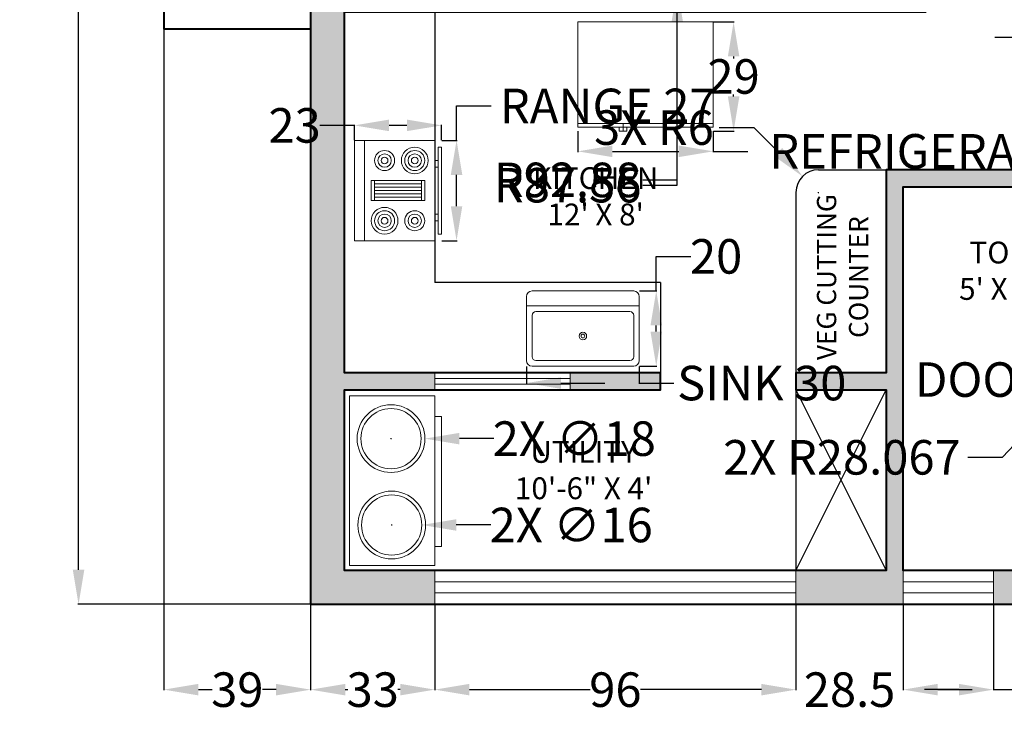
# Model space of a CAD drawing. Units: inches. Extents: x -51 to 563, y -59 to 453.
# Tile 1 of 6: x -51 to 211, y -59 to 125. Entities that reach past the tile are written whole.
import ezdxf

# ---------------------------------------------------------------- set-up
doc = ezdxf.new("R2010")
doc.units = ezdxf.units.IN
doc.header["$MEASUREMENT"] = 0
for name, color, linetype, lineweight in [('A-ANNO-DIMS', 2, 'Continuous', 18), ('A-ANNO-TEXT', 7, 'Continuous', 18), ('A-AREA-IDEN', 7, 'Continuous', 25), ('A-EQPM', 8, 'Continuous', 18), ('A-FLOR-CASE', 8, 'Continuous', 25), ('A-FLOR-FIXT', 9, 'Continuous', 18), ('A-GLAZ', 4, 'Continuous', 18), ('A-WALL', 7, 'Continuous', 40), ('A-WALL-PATT', 252, 'Continuous', 13)]:
    doc.layers.add(name, color=color, linetype=linetype, lineweight=lineweight)
doc.styles.get("Standard").update_dxf_attribs({"font": 'arial.ttf'})
doc.dimstyles.get("Standard").update_dxf_attribs({"dimtxt": 9.18, "dimasz": 9.18, "dimexe": 0.18, "dimexo": 0.0625, "dimgap": 0.09, "dimtad": 0, "dimtih": 1, "dimtoh": 1, "dimdec": 1, "dimzin": 0, "dimdsep": 46, "dimlunit": 3, "dimtxsty": 'Standard', "dimcen": 0.09, "dimadec": 0, "dimazin": 0, "dimtfac": 1, "dimtdec": 1, "dimtofl": 0, "dimtmove": 0, "dimatfit": 3, "dimfxl": 1, "dimtolj": 1, "dimtzin": 0, "dimarcsym": 0})

# ---------------------------------------------------------------- blocks, each defined once
blk = doc.blocks.new('Range-Oven - 30 in top')
for p, q in [((0, -3), (30, -3)), ((12, -6), (18, -6)), ((13, -20), (13, -6)), ((14, -6), (14, -20)), ((15, -20), (15, -6)), ((16, -6), (16, -20)), ((17, -20), (17, -6)), ((18, -20), (12, -20)), ((6, -24), (6, -25)), ((8, -25), (8, -24)), ((22, -25), (22, -24)), ((24, -24), (24, -25))]:
    blk.add_line(p, q)
for points in [[(0, -24), (0, 0), (30, 0), (30, -24)], [(12, -21), (12, -5), (18, -5), (18, -21)], [(2, -26), (2, -25), (28, -25), (28, -26)]]:
    blk.add_lwpolyline(points, close=True)
for centre, radius in [((6, -9), 4), ((6, -9), 3), ((6, -9), 2), ((6, -9), 1), ((24, -9), 3), ((24, -9), 2), ((24, -9), 1), ((24, -18), 4), ((6, -18), 3), ((6, -18), 2), ((6, -18), 1), ((24, -18), 3), ((24, -18), 2), ((24, -18), 1)]:
    blk.add_circle(centre, radius)
blk = doc.blocks.new('Sink-single - 30 in top')
blk.add_line((-15, -3.999996), (15, -3.999996))
for points in [[(-13.5, 0), (13.5, 0)], [(-15, -18.499996), (-15, -1.5)], [(15, -1.5), (15, -18.499996)], [(-13.5, -17.499996), (-13.5, -6.499996)], [(-12.5, -5.499996), (12.5, -5.499996)], [(13.5, -6.499996), (13.5, -17.499996)], [(13.5, -19.999996), (-13.5, -19.999996)], [(12.5, -18.499996), (-12.5, -18.499996)]]:
    blk.add_lwpolyline(points)
for radius in [1, 0.5]:
    blk.add_circle((0, -11.999996), radius)
for centre, radius, start, end in [((-13.5, -1.5), 1.5, 90, 180), ((13.5, -1.5), 1.5, 0, 90), ((-12.5, -6.499996), 1, 90, 180), ((12.5, -6.499996), 1, 0, 90), ((-12.5, -17.499996), 1, 180, 270), ((12.5, -17.499996), 1, 270, 0), ((-13.5, -18.499996), 1.5, 180, 270), ((13.5, -18.499996), 1.5, 270, 0)]:
    blk.add_arc(centre, radius, start, end)
blk = doc.blocks.new('Refrigerator-2 door - 36 in top')
for p, q in [((0, -26.999999), (36, -26.999999)), ((11, -27.999999), (11, -28.999999)), ((12, -26.999999), (12, -28.999999)), ((13, -28.999999), (13, -27.999999)), ((11, -28.999999), (13, -28.999999))]:
    blk.add_line(p, q)
blk.add_lwpolyline([(0, -27.999999), (0, 0), (36, 0), (36, -27.999999)], close=True)
blk = doc.blocks.new('*D43')
at = {"layer": 'A-ANNO-DIMS', "color": 0, "lineweight": -2, "transparency": 16777216}
for p, q in [((244.12, 44.35), (248.82, 44.35)), ((248.64, 35.17), (248.64, 33.92)), ((248.64, 22.99), (248.64, 24.24)), ((244.12, 13.81), (248.82, 13.81))]:
    blk.add_line(p, q, dxfattribs=at)
at = {"layer": 'A-ANNO-DIMS', "color": 0, "transparency": 16777216}
for points in [[(247.11, 35.17), (250.17, 35.17), (248.64, 44.35)], [(247.11, 22.99), (250.17, 22.99), (248.64, 13.81)]]:
    blk.add_solid(points, dxfattribs=at)
at = {"layer": 'Defpoints', "color": 0, "transparency": 16777216}
for p in [(244.06, 44.35), (248.64, 44.35), (244.06, 13.81)]:
    blk.add_point(p, dxfattribs=at)
at = {"layer": 'A-ANNO-DIMS', "color": 0, "transparency": 16777216, "insert": (248.64, 29.08), "char_height": 9.18, "attachment_point": 5}
blk.add_mtext('\\A1;DOOR SWING 31 TYP.', dxfattribs=at)
blk = doc.blocks.new('*D50')
at = {"layer": 'A-ANNO-DIMS', "color": 0, "lineweight": -2, "transparency": 16777216}
for p, q in [((217.6, 120.04), (208.42, 120.04)), ((226.78, 117.06), (226.78, 120.22)), ((243.37, 117.06), (243.37, 120.22)), ((252.55, 120.04), (261.73, 120.04))]:
    blk.add_line(p, q, dxfattribs=at)
at = {"layer": 'A-ANNO-DIMS', "color": 0, "transparency": 16777216}
for points in [[(217.6, 121.57), (217.6, 118.51), (226.78, 120.04)], [(252.55, 121.57), (252.55, 118.51), (243.37, 120.04)]]:
    blk.add_solid(points, dxfattribs=at)
at = {"layer": 'Defpoints', "color": 0, "transparency": 16777216}
for p in [(226.78, 120.04), (226.78, 117), (243.37, 117)]:
    blk.add_point(p, dxfattribs=at)
at = {"layer": 'A-ANNO-DIMS', "color": 0, "transparency": 16777216, "insert": (235.08, 120.04), "char_height": 9.18, "attachment_point": 5}
blk.add_mtext('\\A1;17', dxfattribs=at)
blk = doc.blocks.new('*D51')
at = {"layer": 'A-ANNO-DIMS', "color": 0, "lineweight": -2, "transparency": 16777216}
for p, q in [((65.34, 92.65), (65.34, 101.83)), ((65.34, 101.83), (74.52, 101.83)), ((61.4, 92.65), (65.52, 92.65)), ((65.34, 75.15), (65.34, 83.47)), ((61.4, 65.97), (65.52, 65.97))]:
    blk.add_line(p, q, dxfattribs=at)
at = {"layer": 'A-ANNO-DIMS', "color": 0, "transparency": 16777216}
for points in [[(63.81, 83.47), (66.87, 83.47), (65.34, 92.65)], [(63.81, 75.15), (66.87, 75.15), (65.34, 65.97)]]:
    blk.add_solid(points, dxfattribs=at)
at = {"layer": 'Defpoints', "color": 0, "transparency": 16777216}
for p in [(61.34, 92.65), (65.34, 92.65), (61.34, 65.97)]:
    blk.add_point(p, dxfattribs=at)
at = {"layer": 'A-ANNO-DIMS', "color": 0, "transparency": 16777216, "insert": (105.53, 101.83), "char_height": 9.18, "attachment_point": 5}
blk.add_mtext('\\A1;RANGE 27', dxfattribs=at)
blk = doc.blocks.new('*D52')
at = {"layer": 'A-ANNO-DIMS', "color": 0, "lineweight": -2, "transparency": 16777216}
for p, q in [((38.21, 96.65), (29.03, 96.65)), ((38.21, 92.71), (38.21, 96.83)), ((52.16, 96.65), (47.39, 96.65)), ((61.34, 92.71), (61.34, 96.83))]:
    blk.add_line(p, q, dxfattribs=at)
at = {"layer": 'A-ANNO-DIMS', "color": 0, "transparency": 16777216}
for points in [[(47.39, 98.18), (47.39, 95.12), (38.21, 96.65)], [(52.16, 98.18), (52.16, 95.12), (61.34, 96.65)]]:
    blk.add_solid(points, dxfattribs=at)
at = {"layer": 'Defpoints', "color": 0, "transparency": 16777216}
for p in [(38.21, 96.65), (38.21, 92.65), (61.34, 92.65)]:
    blk.add_point(p, dxfattribs=at)
at = {"layer": 'A-ANNO-DIMS', "color": 0, "transparency": 16777216, "insert": (22.29, 96.65), "char_height": 9.18, "attachment_point": 5}
blk.add_mtext('\\A1;23', dxfattribs=at)
blk = doc.blocks.new('*D53')
at = {"layer": 'A-ANNO-DIMS', "color": 0, "lineweight": -2, "transparency": 16777216}
for p, q in [((83.92, 32.59), (83.92, 27.97)), ((113.92, 32.59), (113.92, 27.97)), ((93.1, 28.15), (104.74, 28.15)), ((113.92, 28.15), (123.1, 28.15))]:
    blk.add_line(p, q, dxfattribs=at)
at = {"layer": 'A-ANNO-DIMS', "color": 0, "transparency": 16777216}
for points in [[(93.1, 29.68), (93.1, 26.62), (83.92, 28.15)], [(104.74, 29.68), (104.74, 26.62), (113.92, 28.15)]]:
    blk.add_solid(points, dxfattribs=at)
at = {"layer": 'Defpoints', "color": 0, "transparency": 16777216}
for p in [(83.92, 32.65), (113.92, 32.65), (113.92, 28.15)]:
    blk.add_point(p, dxfattribs=at)
at = {"layer": 'A-ANNO-DIMS', "color": 0, "transparency": 16777216, "insert": (146.48, 28.15), "char_height": 9.18, "attachment_point": 5}
blk.add_mtext('\\A1;SINK 30', dxfattribs=at)
blk = doc.blocks.new('*D54')
at = {"layer": 'A-ANNO-DIMS', "color": 0, "lineweight": -2, "transparency": 16777216}
for p, q in [((118.42, 52.65), (118.42, 61.83)), ((118.42, 61.83), (127.6, 61.83)), ((113.98, 52.65), (118.6, 52.65)), ((118.42, 41.83), (118.42, 43.47)), ((113.98, 32.65), (118.6, 32.65))]:
    blk.add_line(p, q, dxfattribs=at)
at = {"layer": 'A-ANNO-DIMS', "color": 0, "transparency": 16777216}
for points in [[(116.89, 43.47), (119.95, 43.47), (118.42, 52.65)], [(116.89, 41.83), (119.95, 41.83), (118.42, 32.65)]]:
    blk.add_solid(points, dxfattribs=at)
at = {"layer": 'Defpoints', "color": 0, "transparency": 16777216}
for p in [(113.92, 52.65), (118.42, 52.65), (113.92, 32.65)]:
    blk.add_point(p, dxfattribs=at)
at = {"layer": 'A-ANNO-DIMS', "color": 0, "transparency": 16777216, "insert": (134.33, 61.83), "char_height": 9.18, "attachment_point": 5}
blk.add_mtext('\\A1;20', dxfattribs=at)
blk = doc.blocks.new('*D55')
at = {"layer": 'A-ANNO-DIMS', "color": 0, "lineweight": -2, "transparency": 16777216}
for p, q in [((97.59, 95.09), (97.59, 89.57)), ((133.59, 95.09), (133.59, 89.57)), ((106.77, 89.75), (124.41, 89.75)), ((133.59, 89.75), (142.77, 89.75))]:
    blk.add_line(p, q, dxfattribs=at)
at = {"layer": 'A-ANNO-DIMS', "color": 0, "transparency": 16777216}
for points in [[(106.77, 91.28), (106.77, 88.22), (97.59, 89.75)], [(124.41, 91.28), (124.41, 88.22), (133.59, 89.75)]]:
    blk.add_solid(points, dxfattribs=at)
at = {"layer": 'Defpoints', "color": 0, "transparency": 16777216}
for p in [(97.59, 95.15), (133.59, 95.15), (133.59, 89.75)]:
    blk.add_point(p, dxfattribs=at)
at = {"layer": 'A-ANNO-DIMS', "color": 0, "transparency": 16777216, "insert": (201.92, 89.75), "char_height": 9.18, "attachment_point": 5}
blk.add_mtext('\\A1;REFRIGERATOR 36', dxfattribs=at)
blk = doc.blocks.new('*D56')
at = {"layer": 'A-ANNO-DIMS', "color": 0, "lineweight": -2, "transparency": 16777216}
for p, q in [((133.65, 124.15), (139.17, 124.15)), ((138.99, 114.97), (138.99, 114.43)), ((138.99, 104.33), (138.99, 104.87)), ((133.65, 95.15), (139.17, 95.15))]:
    blk.add_line(p, q, dxfattribs=at)
at = {"layer": 'A-ANNO-DIMS', "color": 0, "transparency": 16777216}
for points in [[(137.46, 114.97), (140.52, 114.97), (138.99, 124.15)], [(137.46, 104.33), (140.52, 104.33), (138.99, 95.15)]]:
    blk.add_solid(points, dxfattribs=at)
at = {"layer": 'Defpoints', "color": 0, "transparency": 16777216}
for p in [(133.59, 124.15), (138.99, 124.15), (133.59, 95.15)]:
    blk.add_point(p, dxfattribs=at)
at = {"layer": 'A-ANNO-DIMS', "color": 0, "transparency": 16777216, "insert": (138.99, 109.65), "char_height": 9.18, "attachment_point": 5}
blk.add_mtext('\\A1;29', dxfattribs=at)
blk = doc.blocks.new('*D66')
at = {"layer": 'A-ANNO-DIMS', "color": 0, "lineweight": -2, "transparency": 16777216}
for p, q in [((26.5, 420.85), (-35.32, 420.85)), ((-35.14, 411.67), (-35.14, 199.87)), ((-35.14, -21.47), (-35.14, 190.32)), ((26.5, -30.65), (-35.32, -30.65))]:
    blk.add_line(p, q, dxfattribs=at)
at = {"layer": 'A-ANNO-DIMS', "color": 0, "transparency": 16777216}
for points in [[(-36.67, 411.67), (-33.61, 411.67), (-35.14, 420.85)], [(-36.67, -21.47), (-33.61, -21.47), (-35.14, -30.65)]]:
    blk.add_solid(points, dxfattribs=at)
at = {"layer": 'Defpoints', "color": 0, "transparency": 16777216}
for p in [(-35.14, 420.85), (26.56, 420.85), (26.56, -30.65)]:
    blk.add_point(p, dxfattribs=at)
at = {"layer": 'A-ANNO-DIMS', "color": 0, "transparency": 16777216, "insert": (-35.14, 195.1), "char_height": 9.18, "attachment_point": 5}
blk.add_mtext('\\A1;451.5', dxfattribs=at)
blk = doc.blocks.new('*D67')
at = {"layer": 'A-ANNO-DIMS', "color": 0, "lineweight": -2, "transparency": 16777216}
for p, q in [((-12.44, 122.29), (-12.44, -53.53)), ((26.56, -30.71), (26.56, -53.53)), ((-3.26, -53.35), (0.39, -53.35)), ((17.38, -53.35), (13.73, -53.35))]:
    blk.add_line(p, q, dxfattribs=at)
at = {"layer": 'A-ANNO-DIMS', "color": 0, "transparency": 16777216}
for points in [[(-3.26, -51.82), (-3.26, -54.88), (-12.44, -53.35)], [(17.38, -51.82), (17.38, -54.88), (26.56, -53.35)]]:
    blk.add_solid(points, dxfattribs=at)
at = {"layer": 'Defpoints', "color": 0, "transparency": 16777216}
for p in [(-12.44, 122.35), (26.56, -30.65), (26.56, -53.35)]:
    blk.add_point(p, dxfattribs=at)
at = {"layer": 'A-ANNO-DIMS', "color": 0, "transparency": 16777216, "insert": (7.06, -53.35), "char_height": 9.18, "attachment_point": 5}
blk.add_mtext('\\A1;39', dxfattribs=at)
blk = doc.blocks.new('*D73')
at = {"layer": 'A-ANNO-DIMS', "color": 0, "lineweight": -2, "transparency": 16777216}
for p, q in [((26.56, -30.71), (26.56, -53.53)), ((59.56, -30.71), (59.56, -53.53)), ((35.74, -53.35), (36.4, -53.35)), ((50.38, -53.35), (49.72, -53.35))]:
    blk.add_line(p, q, dxfattribs=at)
at = {"layer": 'A-ANNO-DIMS', "color": 0, "transparency": 16777216}
for points in [[(35.74, -51.82), (35.74, -54.88), (26.56, -53.35)], [(50.38, -51.82), (50.38, -54.88), (59.56, -53.35)]]:
    blk.add_solid(points, dxfattribs=at)
at = {"layer": 'Defpoints', "color": 0, "transparency": 16777216}
for p in [(26.56, -30.65), (59.56, -30.65), (59.56, -53.35)]:
    blk.add_point(p, dxfattribs=at)
at = {"layer": 'A-ANNO-DIMS', "color": 0, "transparency": 16777216, "insert": (43.06, -53.35), "char_height": 9.18, "attachment_point": 5}
blk.add_mtext('\\A1;33', dxfattribs=at)
blk = doc.blocks.new('*D74')
at = {"layer": 'A-ANNO-DIMS', "color": 0, "lineweight": -2, "transparency": 16777216}
for p, q in [((59.56, -30.71), (59.56, -53.53)), ((155.56, -30.71), (155.56, -53.53)), ((68.74, -53.35), (100.9, -53.35)), ((146.38, -53.35), (114.22, -53.35))]:
    blk.add_line(p, q, dxfattribs=at)
at = {"layer": 'A-ANNO-DIMS', "color": 0, "transparency": 16777216}
for points in [[(68.74, -51.82), (68.74, -54.88), (59.56, -53.35)], [(146.38, -51.82), (146.38, -54.88), (155.56, -53.35)]]:
    blk.add_solid(points, dxfattribs=at)
at = {"layer": 'Defpoints', "color": 0, "transparency": 16777216}
for p in [(59.56, -30.65), (155.56, -30.65), (155.56, -53.35)]:
    blk.add_point(p, dxfattribs=at)
at = {"layer": 'A-ANNO-DIMS', "color": 0, "transparency": 16777216, "insert": (107.56, -53.35), "char_height": 9.18, "attachment_point": 5}
blk.add_mtext('\\A1;96', dxfattribs=at)
blk = doc.blocks.new('*D75')
at = {"layer": 'A-ANNO-DIMS', "color": 0, "lineweight": -2, "transparency": 16777216}
for p, q in [((155.558368, -30.714601), (155.558368, -53.532101)), ((184.058368, -30.714601), (184.058368, -53.532101)), ((146.378368, -53.352101), (137.198368, -53.352101)), ((193.238368, -53.352101), (202.418368, -53.352101))]:
    blk.add_line(p, q, dxfattribs=at)
at = {"layer": 'A-ANNO-DIMS', "color": 0, "transparency": 16777216}
for points in [[(146.378368, -51.822101), (146.378368, -54.882101), (155.558368, -53.352101)], [(193.238368, -51.822101), (193.238368, -54.882101), (184.058368, -53.352101)]]:
    blk.add_solid(points, dxfattribs=at)
at = {"layer": 'Defpoints', "color": 0, "transparency": 16777216}
for p in [(155.558368, -30.652101), (184.058368, -30.652101), (184.058368, -53.352101)]:
    blk.add_point(p, dxfattribs=at)
at = {"layer": 'A-ANNO-DIMS', "color": 0, "transparency": 16777216, "insert": (169.808368, -53.352101), "char_height": 9.18, "attachment_point": 5}
blk.add_mtext('\\A1;28.5', dxfattribs=at)
blk = doc.blocks.new('*D76')
at = {"layer": 'A-ANNO-DIMS', "color": 0, "lineweight": -2, "transparency": 16777216}
for p, q in [((184.06, -30.71), (184.06, -53.53)), ((208.06, -30.71), (208.06, -53.53)), ((193.24, -53.35), (198.88, -53.35)), ((208.06, -53.35), (217.24, -53.35))]:
    blk.add_line(p, q, dxfattribs=at)
at = {"layer": 'A-ANNO-DIMS', "color": 0, "transparency": 16777216}
for points in [[(193.24, -51.82), (193.24, -54.88), (184.06, -53.35)], [(198.88, -51.82), (198.88, -54.88), (208.06, -53.35)]]:
    blk.add_solid(points, dxfattribs=at)
at = {"layer": 'Defpoints', "color": 0, "transparency": 16777216}
for p in [(184.06, -30.65), (208.06, -30.65), (208.06, -53.35)]:
    blk.add_point(p, dxfattribs=at)
at = {"layer": 'A-ANNO-DIMS', "color": 0, "transparency": 16777216, "insert": (223.96, -53.35), "char_height": 9.18, "attachment_point": 5}
blk.add_mtext('\\A1;24', dxfattribs=at)
blk = doc.blocks.new('*D77')
at = {"layer": 'A-ANNO-DIMS', "color": 0, "lineweight": -2, "transparency": 16777216}
for p, q in [((208.058368, -30.714601), (208.058368, -53.532101)), ((248.558368, -30.714601), (248.558368, -53.532101)), ((198.878368, -53.352101), (189.698368, -53.352101)), ((257.738368, -53.352101), (266.918368, -53.352101))]:
    blk.add_line(p, q, dxfattribs=at)
at = {"layer": 'A-ANNO-DIMS', "color": 0, "transparency": 16777216}
for points in [[(198.878368, -51.822101), (198.878368, -54.882101), (208.058368, -53.352101)], [(257.738368, -51.822101), (257.738368, -54.882101), (248.558368, -53.352101)]]:
    blk.add_solid(points, dxfattribs=at)
at = {"layer": 'Defpoints', "color": 0, "transparency": 16777216}
for p in [(208.058368, -30.652101), (248.558368, -30.652101), (248.558368, -53.352101)]:
    blk.add_point(p, dxfattribs=at)
at = {"layer": 'A-ANNO-DIMS', "color": 0, "transparency": 16777216, "insert": (228.308368, -53.352101), "char_height": 9.18, "attachment_point": 5}
blk.add_mtext('\\A1;40.5', dxfattribs=at)
blk = doc.blocks.new('*D85')
at = {"layer": 'A-ANNO-DIMS', "color": 0, "lineweight": -2, "transparency": 16777216}
for p, q in [((242.04, 42.35), (242.22, 42.35)), ((242.13, 42.26), (242.13, 42.44)), ((210.45, 8.41), (216.71, 15.12)), ((201.27, 8.41), (210.45, 8.41))]:
    blk.add_line(p, q, dxfattribs=at)
at = {"layer": 'A-ANNO-DIMS', "color": 0, "transparency": 16777216}
blk.add_solid([(215.59, 16.16), (217.83, 14.07), (222.97, 21.83)], dxfattribs=at)
at = {"layer": 'Defpoints', "color": 0, "transparency": 16777216}
for p in [(242.13, 42.35), (222.97, 21.83)]:
    blk.add_point(p, dxfattribs=at)
at = {"layer": 'A-ANNO-DIMS', "color": 0, "transparency": 16777216, "insert": (167.79, 8.41), "char_height": 9.18, "attachment_point": 5}
blk.add_mtext('\\A1;2X R28.067', dxfattribs=at)
blk = doc.blocks.new('*D86')
at = {"layer": 'A-ANNO-DIMS', "color": 0, "lineweight": -2, "transparency": 16777216}
for p, q in [((47.83, 13.38), (48.01, 13.38)), ((47.92, 13.29), (47.92, 13.47)), ((75.28, 13.38), (66.1, 13.38))]:
    blk.add_line(p, q, dxfattribs=at)
at = {"layer": 'A-ANNO-DIMS', "color": 0, "transparency": 16777216}
blk.add_solid([(66.1, 14.91), (66.1, 11.85), (56.92, 13.38)], dxfattribs=at)
at = {"layer": 'Defpoints', "color": 0, "transparency": 16777216}
for p in [(38.92, 13.38), (56.92, 13.38)]:
    blk.add_point(p, dxfattribs=at)
at = {"layer": 'A-ANNO-DIMS', "color": 0, "transparency": 16777216, "insert": (96.64, 13.38), "char_height": 9.18, "attachment_point": 5}
blk.add_mtext('\\A1;2X ∅18', dxfattribs=at)
blk = doc.blocks.new('*D87')
at = {"layer": 'A-ANNO-DIMS', "color": 0, "lineweight": -2, "transparency": 16777216}
for p, q in [((48.01, -9.58), (48.19, -9.58)), ((48.1, -9.67), (48.1, -9.49)), ((74.46, -9.58), (65.28, -9.58))]:
    blk.add_line(p, q, dxfattribs=at)
at = {"layer": 'A-ANNO-DIMS', "color": 0, "transparency": 16777216}
blk.add_solid([(65.28, -8.05), (65.28, -11.11), (56.1, -9.58)], dxfattribs=at)
at = {"layer": 'Defpoints', "color": 0, "transparency": 16777216}
for p in [(40.1, -9.58), (56.1, -9.58)]:
    blk.add_point(p, dxfattribs=at)
at = {"layer": 'A-ANNO-DIMS', "color": 0, "transparency": 16777216, "insert": (95.82, -9.58), "char_height": 9.18, "attachment_point": 5}
blk.add_mtext('\\A1;2X ∅16', dxfattribs=at)
blk = doc.blocks.new('*D88')
at = {"layer": 'A-ANNO-DIMS', "color": 0, "lineweight": -2, "transparency": 16777216}
for p, q in [((135.15, 96.07), (144.33, 96.07)), ((144.33, 96.07), (150.83, 89.58)), ((161.47, 78.85), (161.65, 78.85)), ((161.56, 78.76), (161.56, 78.94))]:
    blk.add_line(p, q, dxfattribs=at)
at = {"layer": 'A-ANNO-DIMS', "color": 0, "transparency": 16777216}
blk.add_solid([(151.91, 90.66), (149.74, 88.5), (157.32, 83.09)], dxfattribs=at)
at = {"layer": 'Defpoints', "color": 0, "transparency": 16777216}
for p in [(157.32, 83.09), (161.56, 78.85)]:
    blk.add_point(p, dxfattribs=at)
at = {"layer": 'A-ANNO-DIMS', "color": 0, "transparency": 16777216, "insert": (117.81, 96.07), "char_height": 9.18, "attachment_point": 5}
blk.add_mtext('\\A1;3X R6', dxfattribs=at)
blk = doc.blocks.new('*D89')
at = {"layer": 'A-ANNO-DIMS', "color": 0, "lineweight": -2, "transparency": 16777216}
for p, q in [((123.92, 230.78), (124.1, 230.78)), ((124.01, 230.69), (124.01, 230.87)), ((124.01, 82.16), (124.01, 128.71)), ((114.83, 82.16), (124.01, 82.16))]:
    blk.add_line(p, q, dxfattribs=at)
at = {"layer": 'A-ANNO-DIMS', "color": 0, "transparency": 16777216}
blk.add_solid([(122.48, 128.71), (125.54, 128.71), (124.01, 137.89)], dxfattribs=at)
at = {"layer": 'Defpoints', "color": 0, "transparency": 16777216}
for p in [(124.01, 230.78), (124.01, 137.89)]:
    blk.add_point(p, dxfattribs=at)
at = {"layer": 'A-ANNO-DIMS', "color": 0, "transparency": 16777216, "insert": (94.85, 82.16), "char_height": 9.18, "attachment_point": 5}
blk.add_mtext('\\A1;R92.88', dxfattribs=at)
blk = doc.blocks.new('*D90')
at = {"layer": 'A-ANNO-DIMS', "color": 0, "lineweight": -2, "transparency": 16777216}
for p, q in [((123.92, 220.85), (124.1, 220.85)), ((124.01, 220.76), (124.01, 220.94)), ((124.01, 80.76), (124.01, 124.11)), ((114.83, 80.76), (124.01, 80.76))]:
    blk.add_line(p, q, dxfattribs=at)
at = {"layer": 'A-ANNO-DIMS', "color": 0, "transparency": 16777216}
blk.add_solid([(122.48, 124.11), (125.54, 124.11), (124.01, 133.29)], dxfattribs=at)
at = {"layer": 'Defpoints', "color": 0, "transparency": 16777216}
for p in [(124.01, 220.85), (124.01, 133.29)]:
    blk.add_point(p, dxfattribs=at)
at = {"layer": 'A-ANNO-DIMS', "color": 0, "transparency": 16777216, "insert": (94.86, 80.76), "char_height": 9.18, "attachment_point": 5}
blk.add_mtext('\\A1;R87.56', dxfattribs=at)

msp = doc.modelspace()

# ---------------------------------------------------------------- linework, layer by layer
at = {"layer": 'A-EQPM'}
for points in [[(36.9265, 24.7375), (59.5584, 24.7375), (59.5584, -20.3368), (36.9265, -20.3368)], [(59.5584, 19.288), (61.3427, 19.288), (61.3427, -15.3158), (59.5584, -15.3158)]]:
    msp.add_lwpolyline(points, close=True, dxfattribs=at)
for centre, radius in [((47.9191, 13.38), 9), ((47.9191, 13.38), 8), ((48.1026, -9.5825), 9), ((48.1026, -9.5825), 8)]:
    msp.add_circle(centre, radius, dxfattribs=at)
at = {"layer": 'A-FLOR-CASE'}
for p, q in [((59.5584, 126.8479), (59.5584, 54.8479)), ((161.5584, 84.8479), (179.5584, 84.8479)), ((155.5584, 78.8479), (155.5584, 30.8479)), ((119.5584, 54.8479), (119.5584, 30.8479)), ((155.5584, 26.3479), (179.5584, -21.6521)), ((155.5584, -21.6521), (179.5584, 26.3479)), ((155.5584, 26.3479), (155.5584, -21.6521))]:
    msp.add_line(p, q, dxfattribs=at)
msp.add_lwpolyline([(119.5584, 54.8479), (59.5584, 54.8479)], dxfattribs=at)
msp.add_arc((161.5584, 78.8479), 6, 90, 180, dxfattribs=at)
at = {"layer": 'A-GLAZ'}
for p, q in [((59.5584, 30.8479), (59.5584, 26.3479)), ((95.5584, 30.8479), (95.5584, 26.3479)), ((59.5584, -21.6521), (59.5584, -30.6521)), ((155.5584, -21.6521), (155.5584, -30.6521)), ((184.0584, -21.6521), (184.0584, -30.6521)), ((208.0584, -21.6521), (208.0584, -30.6521))]:
    msp.add_line(p, q, dxfattribs=at)
for points in [[(95.5584, 29.3479), (59.5584, 29.3479)], [(95.5584, 27.8479), (59.5584, 27.8479)], [(155.5584, -24.6521), (59.5584, -24.6521)], [(208.0584, -24.6521), (184.0584, -24.6521)], [(155.5584, -27.6521), (59.5584, -27.6521)], [(208.0584, -27.6521), (184.0584, -27.6521)]]:
    msp.add_lwpolyline(points, dxfattribs=at)
at = {"layer": 'A-WALL'}
for points in [[(422.5584, 420.8479), (26.5584, 420.8479), (26.5584, 267.8479), (26.5584, 263.3479), (35.5584, 263.3479), (50.5584, 263.3479), (50.5584, 131.3479), (35.5584, 131.3479), (26.5584, 131.3479), (26.5584, 126.8479), (26.5584, 0.8479), (26.5584, -30.6521), (35.5584, -30.6521), (284.5584, -30.6521)], [(26.5584, 272.3479), (-9.4416, 272.3479), (-12.4416, 272.3479), (-12.4416, 267.8479), (-12.4416, 126.8479), (-12.4416, 122.3479), (-9.4416, 122.3479), (26.5584, 122.3479)], [(244.0584, 84.8479), (179.5584, 84.8479), (179.5584, 30.8479), (155.5584, 30.8479), (155.5584, 26.3479), (179.5584, 26.3479), (179.5584, -21.6521), (35.5584, -21.6521), (35.5584, 26.3479), (119.5584, 26.3479), (119.5584, 30.8479), (35.5584, 30.8479), (35.5584, 126.8479), (190.0584, 126.8479), (190.0584, 131.3479), (59.5584, 131.3479), (59.5584, 263.3479)], [(244.0584, -21.6521), (184.0584, -21.6521), (184.0584, 80.3479), (244.0584, 80.3479)]]:
    msp.add_lwpolyline(points, dxfattribs=at)
at = {"layer": 'A-WALL-PATT'}
for points in [[(26.5584, 131.3479), (35.5584, 126.8479), (26.5584, -30.6521), (35.5584, -21.6521)], [(184.0584, -30.6521), (179.5584, -21.6521), (184.0584, 80.3479), (179.5584, 84.8479)], [(184.0584, 80.3479), (179.5584, 84.8479), (244.0584, 80.3479), (244.0584, 84.8479)], [(35.5584, 30.8479), (35.5584, 26.3479), (59.5584, 30.8479), (59.5584, 26.3479)], [(95.5584, 30.8479), (95.5584, 26.3479), (119.5584, 30.8479), (119.5584, 26.3479)], [(155.5584, 30.8479), (155.5584, 26.3479), (179.5584, 30.8479), (179.5584, 26.3479)], [(26.5584, -30.6521), (35.5584, -21.6521), (59.5584, -30.6521), (59.5584, -21.6521)], [(155.5584, -30.6521), (155.5584, -21.6521), (184.0584, -30.6521), (179.5584, -21.6521)], [(208.0584, -21.6521), (208.0584, -30.6521), (244.0584, -21.6521), (248.5584, -30.6521)]]:
    msp.add_solid(points, dxfattribs=at)

# ---------------------------------------------------------------- block references
at = {"layer": 'A-EQPM'}
msp.add_blockref('Refrigerator-2 door - 36 in top', (97.5864, 124.1492), dxfattribs=at)
at = {"layer": 'A-EQPM', "xscale": 0.8894441410229298, "yscale": 0.8894441410229298, "zscale": 0.8894441410229298, "rotation": 90}
msp.add_blockref('Range-Oven - 30 in top', (38.2117, 65.9687), dxfattribs=at)
at = {"layer": 'A-FLOR-FIXT'}
msp.add_blockref('Sink-single - 30 in top', (98.9213, 52.6528), dxfattribs=at)

# ---------------------------------------------------------------- texts
at = {"layer": 'A-ANNO-TEXT', "insert": (161.1482, 30.8479), "char_height": 5.103584, "attachment_point": 1, "rotation": 90}
msp.add_mtext_dynamic_manual_height_columns('\\pxqc;VEG CUTTING COUNTER', width=50.958184, gutter_width=0.8799, heights=[0], dxfattribs=at)
at = {"layer": 'A-AREA-IDEN', "char_height": 5.8, "attachment_point": 1}
for s, width, insert in [("\\pxqc;KITCHEN\\P12' X 8'", 38.109094, (83.253, 85.5309)), ('\\pxqc;TOILET\\P5\' X 8\'-6"', 49.588896, (190.204, 65.7447)), ('\\pxqc;UTILITY\\P10\'-6" X 4\'', 36.674117, (80.7741, 12.7503))]:
    msp.add_mtext_dynamic_manual_height_columns(s, width=width, gutter_width=1, heights=[0], dxfattribs=dict(at, insert=insert))

# ---------------------------------------------------------------- dimensions: what is measured, and where the dimension line sits
at = {"layer": 'A-ANNO-DIMS'}
for base, p1, p2, angle, override, picture, middle in [((-35.1416, 420.8479), (26.5584, -30.6521), (26.5584, 420.8479), 90, {"dimdec": 1, "dimlfac": 1, "dimrnd": 0, "dimzin": 0, "dimdsep": 46, "dimlunit": 2}, '*D66', (-35.1416, 195.0979)), ((226.7786, 120.0365), (243.3723, 117.0018), (226.7786, 117.0018), 180, {"dimdec": 0, "dimlfac": 1, "dimrnd": 0, "dimzin": 0, "dimdsep": 46, "dimlunit": 2}, '*D50', (235.0754, 120.0365)), ((138.9864, 124.1492), (133.5864, 95.1492), (133.5864, 124.1492), 90, {"dimdec": 0, "dimlfac": 1, "dimrnd": 0, "dimzin": 0, "dimdsep": 46, "dimlunit": 2}, '*D56', (138.9864, 109.6492)), ((38.2117, 96.6545), (61.3373, 92.652), (38.2117, 92.652), 180, {"dimdec": 0, "dimlfac": 1, "dimrnd": 0, "dimzin": 0, "dimdsep": 46, "dimlunit": 2}, '*D52', (22.2884, 96.6545)), ((118.4213, 52.6528), (113.9213, 32.6528), (113.9213, 52.6528), 90, {"dimdec": 0, "dimlfac": 1, "dimrnd": 0, "dimzin": 0, "dimdsep": 46, "dimlunit": 2}, '*D54', (134.3289, 61.8328))]:
    dim = msp.add_linear_dim(base=base, p1=p1, p2=p2, angle=angle, dimstyle='Standard', override=override, dxfattribs=at)
    dim.commit()
    dim.dimension.update_dxf_attribs({"geometry": picture, "text_midpoint": middle})
for center, mpoint, picture, middle in [((124.0132, 230.7757), (124.013, 137.8928), '*D89', (94.8518, 82.163)), ((124.0132, 220.8536), (124.013, 133.2945), '*D90', (94.8644, 80.759))]:
    dim = msp.add_radius_dim(center=center, mpoint=mpoint, dimstyle='Standard', override={"dimdec": 2, "dimlfac": 1, "dimrnd": 0, "dimzin": 0, "dimdsep": 46, "dimlunit": 2}, dxfattribs=at)
    dim.commit()
    dim.dimension.update_dxf_attribs({"geometry": picture, "text_midpoint": middle, "dimtype": 164})
for base, p1, p2, override, picture, middle in [((26.5584, -53.3521), (-12.4416, 122.3479), (26.5584, -30.6521), {"dimdec": 0, "dimlfac": 1, "dimrnd": 0, "dimzin": 0, "dimdsep": 46, "dimlunit": 2}, '*D67', (7.0584, -53.3521)), ((59.5584, -53.3521), (26.5584, -30.6521), (59.5584, -30.6521), {"dimdec": 0, "dimlfac": 1, "dimrnd": 0, "dimzin": 0, "dimdsep": 46, "dimlunit": 2}, '*D73', (43.0584, -53.3521)), ((155.5584, -53.3521), (59.5584, -30.6521), (155.5584, -30.6521), {"dimdec": 0, "dimlfac": 1, "dimrnd": 0, "dimzin": 0, "dimdsep": 46, "dimlunit": 2}, '*D74', (107.5584, -53.3521)), ((184.0584, -53.3521), (155.5584, -30.6521), (184.0584, -30.6521), {"dimdec": 1, "dimlfac": 1, "dimrnd": 0, "dimzin": 0, "dimdsep": 46, "dimlunit": 2}, '*D75', (169.8084, -53.3521)), ((208.0584, -53.3521), (184.0584, -30.6521), (208.0584, -30.6521), {"dimdec": 0, "dimlfac": 1, "dimrnd": 0, "dimzin": 0, "dimdsep": 46, "dimlunit": 2}, '*D76', (223.9629, -53.3521)), ((248.5584, -53.3521), (208.0584, -30.6521), (248.5584, -30.6521), {"dimdec": 1, "dimlfac": 1, "dimrnd": 0, "dimzin": 0, "dimdsep": 46, "dimlunit": 2}, '*D77', (228.3084, -53.3521))]:
    dim = msp.add_linear_dim(base=base, p1=p1, p2=p2, dimstyle='Standard', override=override, dxfattribs=at)
    dim.commit()
    dim.dimension.update_dxf_attribs({"geometry": picture, "text_midpoint": middle})
for base, p1, p2, text, picture, middle in [((65.3398, 92.652), (61.3373, 65.9687), (61.3373, 92.652), 'RANGE <>', '*D51', (105.5312, 101.832)), ((248.6388, 44.3479), (244.0584, 13.812), (244.0584, 44.3479), 'DOOR SWING <> TYP.', '*D43', (248.6388, 29.08))]:
    dim = msp.add_linear_dim(base=base, p1=p1, p2=p2, angle=90, text=text, dimstyle='Standard', override={"dimdec": 0, "dimlfac": 1, "dimrnd": 0, "dimzin": 0, "dimdsep": 46, "dimlunit": 2}, dxfattribs=at)
    dim.commit()
    dim.dimension.update_dxf_attribs({"geometry": picture, "text_midpoint": middle})
for center, mpoint, text, override, picture, middle in [((161.5584, 78.8479), (157.3161, 83.0909), '3X <>', {"dimdec": 0, "dimlfac": 1, "dimrnd": 0, "dimzin": 0, "dimdsep": 46, "dimlunit": 2}, '*D88', (117.8068, 96.0745)), ((242.125, 42.3479), (222.9746, 21.8296), '2X <>', {"dimdec": 3, "dimlfac": 1, "dimrnd": 0, "dimzin": 0, "dimdsep": 46, "dimlunit": 2}, '*D85', (167.7886, 8.4074))]:
    dim = msp.add_radius_dim(center=center, mpoint=mpoint, text=text, dimstyle='Standard', override=override, dxfattribs=at)
    dim.commit()
    dim.dimension.update_dxf_attribs({"geometry": picture, "text_midpoint": middle})
for base, p1, p2, text, picture, middle in [((133.5864, 89.7492), (97.5864, 95.1492), (133.5864, 95.1492), 'REFRIGERATOR <>', '*D55', (201.9159, 89.7492)), ((113.9213, 28.1528), (83.9213, 32.6528), (113.9213, 32.6528), 'SINK <>', '*D53', (146.4763, 28.1528))]:
    dim = msp.add_linear_dim(base=base, p1=p1, p2=p2, text=text, dimstyle='Standard', override={"dimdec": 0, "dimlfac": 1, "dimrnd": 0, "dimzin": 0, "dimdsep": 46, "dimlunit": 2}, dxfattribs=at)
    dim.commit()
    dim.dimension.update_dxf_attribs({"geometry": picture, "text_midpoint": middle})
for p1, p2, picture, middle in [((38.9191, 13.3801), (56.9191, 13.38), '*D86', (75.2791, 13.3799)), ((40.1026, -9.583), (56.1026, -9.582), '*D87', (74.4626, -9.5809))]:
    dim = msp.add_diameter_dim_2p(p1=p1, p2=p2, text='2X <>', dimstyle='Standard', override={"dimdec": 0, "dimlfac": 1, "dimrnd": 0, "dimzin": 0, "dimdsep": 46, "dimlunit": 2}, dxfattribs=at)
    dim.commit()
    dim.dimension.update_dxf_attribs({"geometry": picture, "text_midpoint": middle, "dimtype": 163})

doc.saveas('drawing.dxf')
